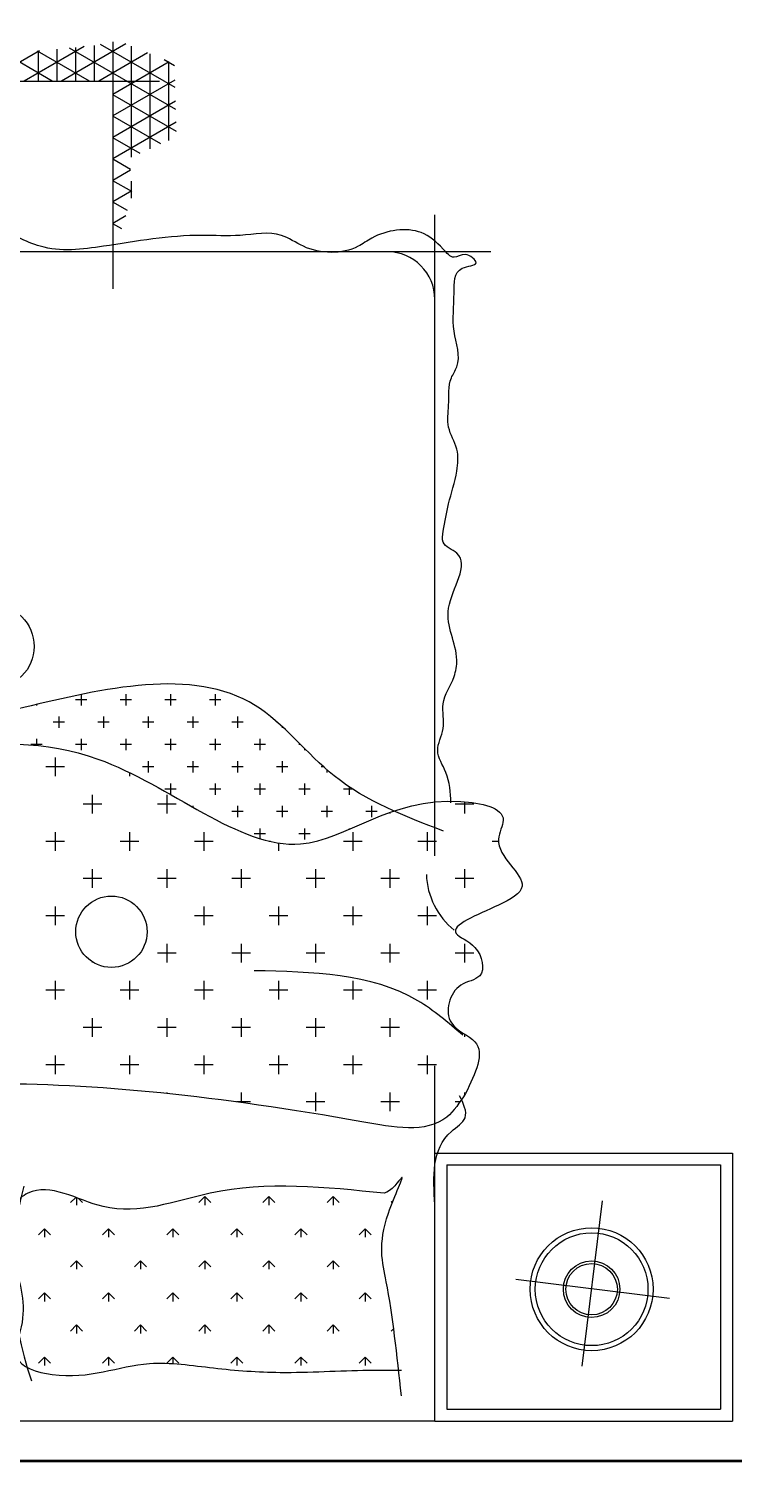
# Model space of a CAD drawing. Units: inches. Extents: x 3731 to 4318, y 1310 to 2388.
# Tile 13 of 57: x 4038 to 4086, y 1363 to 1463. Entities that reach past the tile are written whole.
import ezdxf

# ---------------------------------------------------------------- set-up
doc = ezdxf.new("R2010")
doc.units = ezdxf.units.IN
for name, color, linetype, lineweight in [('A-ANNO-DIMS', 2, 'Continuous', 18), ('A-FURN', 8, 'Continuous', 13), ('A-WALL', 7, 'Continuous', 35)]:
    doc.layers.add(name, color=color, linetype=linetype, lineweight=lineweight)
doc.styles.get("Standard").update_dxf_attribs({"font": 'arial.ttf'})
doc.dimstyles.get("Standard").update_dxf_attribs({"dimtxt": 0.18, "dimasz": 0.18, "dimexe": 0.18, "dimexo": 0.0625, "dimgap": 0.09, "dimtad": 0, "dimtih": 1, "dimtoh": 1, "dimdec": 4, "dimzin": 0, "dimdsep": 46, "dimtxsty": 'Standard', "dimcen": 0.09, "dimadec": 0, "dimazin": 0, "dimtfac": 1, "dimtdec": 4, "dimtofl": 0, "dimtmove": 0, "dimatfit": 3, "dimfxl": 1, "dimtolj": 1, "dimtzin": 0, "dimarcsym": 0})

# ---------------------------------------------------------------- blocks, each defined once
blk = doc.blocks.new('A$C200C7901')
for p, q in [((0, 1.8834), (0, 2.3334)), ((0.5, 2.3334), (0, 2.3334)), ((0.5, 2.3334), (0.5, 1.7369)), ((0.5, 2.3334), (0.5, 1.7369)), ((0.5, 2.3334), (2, 2.3334)), ((0.9943, 2.1721), (0.9842, 2.1822)), ((0.9943, 2.1721), (0.9842, 2.1822)), ((0.9943, 2.0643), (0.9842, 2.0744)), ((0.9943, 2.0643), (0.9842, 2.0744)), ((0.5701, 1.9635), (0.5733, 1.9666)), ((0.5701, 1.9635), (0.5733, 1.9666)), ((0.5, 1.8834), (0, 1.8834)), ((0.4504, 1.782), (0.4504, 1.7863)), ((0.4504, 1.782), (0.4504, 1.7863)), ((0.458, 1.7977), (0.466, 1.7977)), ((0.458, 1.7977), (0.466, 1.7977)), ((1.1222, 1.7352), (1.1535, 1.7352)), ((1.1379, 1.7195), (1.1379, 1.7508)), ((0.4504, 1.6834), (0.4504, 1.6883)), ((0.4504, 1.6834), (0.4504, 1.6883)), ((0.4656, 1.6727), (0.466, 1.6727)), ((0.4656, 1.6727), (0.466, 1.6727)), ((0.5597, 1.6727), (0.591, 1.6727)), ((0.5597, 1.6727), (0.591, 1.6727)), ((1.0129, 1.5945), (1.0129, 1.6258)), ((1.0129, 1.5945), (1.0129, 1.6258)), ((0.4504, 1.532), (0.4504, 1.5633)), ((1.0754, 1.5625), (1.0754, 1.5633)), ((1.0754, 1.5625), (1.0754, 1.5633)), ((0.4347, 1.5477), (0.466, 1.5477)), ((0.6847, 1.5477), (0.716, 1.5477)), ((0.4347, 1.4227), (0.466, 1.4227)), ((0.5, 1.3845), (0.5, 0.3086)), ((0.3931, 1.3602), (0.4035, 1.3602)), ((0.3931, 1.3602), (0.4035, 1.3602)), ((0.4972, 1.3602), (0.5285, 1.3602)), ((0.4972, 1.3602), (0.5285, 1.3602)), ((0.4347, 1.2977), (0.466, 1.2977)), ((0.4347, 1.2977), (0.466, 1.2977)), ((0.4504, 1.2936), (0.4504, 1.3133)), ((0.4504, 1.2936), (0.4504, 1.3133)), ((1.0407, 0.0275), (1.0407, 0.4323)), ((0.4061, 0.3703), (2.0386, 0.3703)), ((2.4073, 0.0839), (0.9625, 0.0839))]:
    blk.add_line(p, q)
at = {"linetype": 'ByBlock'}
for p, q in [((0.02, 1.9034), (0.02, 2.3134)), ((0.48, 2.3134), (0.02, 2.3134)), ((0.48, 1.9034), (0.48, 2.3134)), ((0.2524, 2.2412), (0.2186, 1.9635)), ((0.6171, 2.2259), (0.607, 2.236)), ((0.6171, 2.2259), (0.607, 2.236)), ((0.6171, 2.2259), (0.6171, 2.2402)), ((0.6171, 2.2259), (0.6171, 2.2402)), ((0.6171, 2.2259), (0.6272, 2.236)), ((0.6171, 2.2259), (0.6272, 2.236)), ((0.7249, 2.2259), (0.7148, 2.236)), ((0.7249, 2.2259), (0.7148, 2.236)), ((0.7249, 2.2259), (0.7249, 2.2402)), ((0.7249, 2.2259), (0.7249, 2.2402)), ((0.7249, 2.2259), (0.735, 2.236)), ((0.7249, 2.2259), (0.735, 2.236)), ((0.8326, 2.2259), (0.8225, 2.236)), ((0.8326, 2.2259), (0.8225, 2.236)), ((0.8326, 2.2259), (0.8326, 2.2402)), ((0.8326, 2.2259), (0.8326, 2.2402)), ((0.8326, 2.2259), (0.8427, 2.236)), ((0.8326, 2.2259), (0.8427, 2.236)), ((0.9404, 2.2259), (0.9303, 2.236)), ((0.9404, 2.2259), (0.9303, 2.236)), ((0.9404, 2.2259), (0.9404, 2.2369)), ((0.9404, 2.2259), (0.9404, 2.2369)), ((0.9404, 2.2259), (0.9505, 2.236)), ((0.9404, 2.2259), (0.9505, 2.236)), ((1.0482, 2.2259), (1.0381, 2.236)), ((1.0482, 2.2259), (1.0381, 2.236)), ((1.0482, 2.2259), (1.0482, 2.2402)), ((1.0482, 2.2259), (1.0482, 2.2402)), ((1.0482, 2.2259), (1.0583, 2.236)), ((1.0482, 2.2259), (1.0583, 2.236)), ((1.1559, 2.2259), (1.1458, 2.236)), ((1.1559, 2.2259), (1.1458, 2.236)), ((1.1559, 2.2259), (1.1559, 2.2402)), ((1.1559, 2.2259), (1.1559, 2.2402)), ((1.1559, 2.2259), (1.166, 2.236)), ((1.1559, 2.2259), (1.166, 2.236)), ((0.5692, 2.178), (0.5733, 2.1822)), ((0.5692, 2.178), (0.5733, 2.1822)), ((0.671, 2.1721), (0.6609, 2.1822)), ((0.671, 2.1721), (0.6609, 2.1822)), ((0.671, 2.172), (0.671, 2.1863)), ((0.671, 2.172), (0.671, 2.1863)), ((0.671, 2.1721), (0.6811, 2.1822)), ((0.671, 2.1721), (0.6811, 2.1822)), ((0.7787, 2.1721), (0.7686, 2.1822)), ((0.7787, 2.1721), (0.7686, 2.1822)), ((0.7787, 2.172), (0.7787, 2.1863)), ((0.7787, 2.172), (0.7787, 2.1863)), ((0.7787, 2.1721), (0.7889, 2.1822)), ((0.7787, 2.1721), (0.7889, 2.1822)), ((0.8865, 2.1721), (0.8764, 2.1822)), ((0.8865, 2.1721), (0.8764, 2.1822)), ((0.8865, 2.172), (0.8865, 2.1863)), ((0.8865, 2.172), (0.8865, 2.1863)), ((0.8865, 2.1721), (0.8966, 2.1822)), ((0.8865, 2.1721), (0.8966, 2.1822)), ((0.9943, 2.172), (0.9943, 2.1863)), ((0.9943, 2.172), (0.9943, 2.1863)), ((0.9943, 2.1721), (1.0044, 2.1822)), ((0.9943, 2.1721), (1.0044, 2.1822)), ((1.102, 2.1721), (1.0919, 2.1822)), ((1.102, 2.1721), (1.0919, 2.1822)), ((1.102, 2.172), (1.102, 2.1863)), ((1.102, 2.172), (1.102, 2.1863)), ((1.102, 2.1721), (1.1121, 2.1822)), ((1.102, 2.1721), (1.1121, 2.1822)), ((0.3641, 2.0951), (0.1061, 2.1268)), ((0.6171, 2.1182), (0.607, 2.1283)), ((0.6171, 2.1182), (0.607, 2.1283)), ((0.6171, 2.1182), (0.6171, 2.1325)), ((0.6171, 2.1182), (0.6171, 2.1325)), ((0.6171, 2.1182), (0.6272, 2.1283)), ((0.6171, 2.1182), (0.6272, 2.1283)), ((0.7249, 2.1182), (0.7148, 2.1283)), ((0.7249, 2.1182), (0.7148, 2.1283)), ((0.7249, 2.1182), (0.7249, 2.1325)), ((0.7249, 2.1182), (0.7249, 2.1325)), ((0.7249, 2.1182), (0.735, 2.1283)), ((0.7249, 2.1182), (0.735, 2.1283)), ((0.8326, 2.1182), (0.8225, 2.1283)), ((0.8326, 2.1182), (0.8225, 2.1283)), ((0.8326, 2.1182), (0.8326, 2.1325)), ((0.8326, 2.1182), (0.8326, 2.1325)), ((0.8326, 2.1182), (0.8427, 2.1283)), ((0.8326, 2.1182), (0.8427, 2.1283)), ((0.9404, 2.1182), (0.9303, 2.1283)), ((0.9404, 2.1182), (0.9303, 2.1283)), ((0.9404, 2.1182), (0.9404, 2.1325)), ((0.9404, 2.1182), (0.9404, 2.1325)), ((0.9404, 2.1182), (0.9505, 2.1283)), ((0.9404, 2.1182), (0.9505, 2.1283)), ((1.0482, 2.1182), (1.0381, 2.1283)), ((1.0482, 2.1182), (1.0381, 2.1283)), ((1.0482, 2.1182), (1.0482, 2.1325)), ((1.0482, 2.1182), (1.0482, 2.1325)), ((1.0482, 2.1182), (1.0583, 2.1283)), ((1.0482, 2.1182), (1.0583, 2.1283)), ((1.1559, 2.1182), (1.1458, 2.1283)), ((1.1559, 2.1182), (1.1458, 2.1283)), ((1.1559, 2.1182), (1.1559, 2.1325)), ((1.1559, 2.1182), (1.1559, 2.1325)), ((1.1559, 2.1182), (1.166, 2.1283)), ((1.1559, 2.1182), (1.166, 2.1283)), ((0.671, 2.0643), (0.671, 2.0786)), ((0.671, 2.0643), (0.671, 2.0786)), ((0.7787, 2.0643), (0.7787, 2.0786)), ((0.7787, 2.0643), (0.7787, 2.0786)), ((0.8865, 2.0643), (0.8865, 2.0786)), ((0.8865, 2.0643), (0.8865, 2.0786)), ((0.9943, 2.0643), (0.9943, 2.0786)), ((0.9943, 2.0643), (0.9943, 2.0786)), ((1.102, 2.0643), (1.102, 2.0786)), ((1.102, 2.0643), (1.102, 2.0786)), ((0.671, 2.0643), (0.6609, 2.0744)), ((0.671, 2.0643), (0.6609, 2.0744)), ((0.671, 2.0643), (0.6811, 2.0744)), ((0.671, 2.0643), (0.6811, 2.0744)), ((0.7787, 2.0643), (0.7686, 2.0744)), ((0.7787, 2.0643), (0.7686, 2.0744)), ((0.7787, 2.0643), (0.7889, 2.0744)), ((0.7787, 2.0643), (0.7889, 2.0744)), ((0.8865, 2.0643), (0.8764, 2.0744)), ((0.8865, 2.0643), (0.8764, 2.0744)), ((0.8865, 2.0643), (0.8966, 2.0744)), ((0.8865, 2.0643), (0.8966, 2.0744)), ((0.9943, 2.0643), (1.0044, 2.0744)), ((0.9943, 2.0643), (1.0044, 2.0744)), ((1.102, 2.0643), (1.0919, 2.0744)), ((1.102, 2.0643), (1.0919, 2.0744)), ((1.102, 2.0643), (1.1121, 2.0744)), ((1.102, 2.0643), (1.1121, 2.0744)), ((0.6171, 2.0104), (0.607, 2.0205)), ((0.6171, 2.0104), (0.607, 2.0205)), ((0.6171, 2.0104), (0.6171, 2.0247)), ((0.6171, 2.0104), (0.6171, 2.0247)), ((0.6171, 2.0104), (0.6272, 2.0205)), ((0.6171, 2.0104), (0.6272, 2.0205)), ((0.7249, 2.0104), (0.7148, 2.0205)), ((0.7249, 2.0104), (0.7148, 2.0205)), ((0.7249, 2.0104), (0.7249, 2.0247)), ((0.7249, 2.0104), (0.7249, 2.0247)), ((0.7249, 2.0104), (0.735, 2.0205)), ((0.7249, 2.0104), (0.735, 2.0205)), ((0.8326, 2.0104), (0.8225, 2.0205)), ((0.8326, 2.0104), (0.8225, 2.0205)), ((0.8326, 2.0104), (0.8326, 2.0247)), ((0.8326, 2.0104), (0.8326, 2.0247)), ((0.8326, 2.0104), (0.8427, 2.0205)), ((0.8326, 2.0104), (0.8427, 2.0205)), ((0.9404, 2.0104), (0.9303, 2.0205)), ((0.9404, 2.0104), (0.9303, 2.0205)), ((0.9404, 2.0104), (0.9404, 2.0247)), ((0.9404, 2.0104), (0.9404, 2.0247)), ((0.9404, 2.0104), (0.9505, 2.0205)), ((0.9404, 2.0104), (0.9505, 2.0205)), ((1.0482, 2.0104), (1.0381, 2.0205)), ((1.0482, 2.0104), (1.0381, 2.0205)), ((1.0482, 2.0104), (1.0482, 2.0247)), ((1.0482, 2.0104), (1.0482, 2.0247)), ((1.0482, 2.0104), (1.0583, 2.0205)), ((1.0482, 2.0104), (1.0583, 2.0205)), ((1.1559, 2.0104), (1.1458, 2.0205)), ((1.1559, 2.0104), (1.1458, 2.0205)), ((1.1559, 2.0104), (1.1559, 2.0247)), ((1.1559, 2.0104), (1.1559, 2.0247)), ((1.1559, 2.0104), (1.166, 2.0205)), ((1.1559, 2.0104), (1.166, 2.0205)), ((0.671, 1.9565), (0.6609, 1.9666)), ((0.671, 1.9565), (0.6609, 1.9666)), ((0.671, 1.9565), (0.671, 1.9708)), ((0.671, 1.9565), (0.671, 1.9708)), ((0.671, 1.9565), (0.6811, 1.9666)), ((0.671, 1.9565), (0.6811, 1.9666)), ((0.7787, 1.9565), (0.7686, 1.9666)), ((0.7787, 1.9565), (0.7686, 1.9666)), ((0.7787, 1.9565), (0.7787, 1.9708)), ((0.7787, 1.9565), (0.7787, 1.9708)), ((0.7787, 1.9565), (0.7889, 1.9666)), ((0.7787, 1.9565), (0.7889, 1.9666)), ((0.8865, 1.9565), (0.8764, 1.9666)), ((0.8865, 1.9565), (0.8764, 1.9666)), ((0.8865, 1.9565), (0.8865, 1.9708)), ((0.8865, 1.9565), (0.8865, 1.9708)), ((0.8865, 1.9565), (0.8966, 1.9666)), ((0.8865, 1.9565), (0.8966, 1.9666)), ((1.0993, 1.9593), (1.0919, 1.9666)), ((1.0993, 1.9593), (1.0919, 1.9666)), ((1.102, 1.9583), (1.102, 1.9708)), ((1.102, 1.9583), (1.102, 1.9708)), ((1.1033, 1.9578), (1.1121, 1.9666)), ((1.1033, 1.9578), (1.1121, 1.9666)), ((0.48, 1.9034), (0.02, 1.9034)), ((0.5754, 1.782), (0.5754, 1.8133)), ((0.5754, 1.782), (0.5754, 1.8133)), ((0.7004, 1.782), (0.7004, 1.8133)), ((0.7004, 1.782), (0.7004, 1.8133)), ((0.5597, 1.7977), (0.591, 1.7977)), ((0.5597, 1.7977), (0.591, 1.7977)), ((0.6847, 1.7977), (0.716, 1.7977)), ((0.6847, 1.7977), (0.716, 1.7977)), ((0.8097, 1.7977), (0.8331, 1.7977)), ((0.8097, 1.7977), (0.8331, 1.7977)), ((0.8254, 1.782), (0.8254, 1.7987)), ((0.8254, 1.782), (0.8254, 1.7987)), ((0.9504, 1.782), (0.9504, 1.7836)), ((0.9504, 1.782), (0.9504, 1.7836)), ((0.4972, 1.7352), (0.5285, 1.7352)), ((0.4972, 1.7352), (0.5285, 1.7352)), ((0.5129, 1.7195), (0.5129, 1.7508)), ((0.5129, 1.7195), (0.5129, 1.7508)), ((0.6222, 1.7352), (0.6535, 1.7352)), ((0.6222, 1.7352), (0.6535, 1.7352)), ((0.6379, 1.7195), (0.6379, 1.7508)), ((0.6379, 1.7195), (0.6379, 1.7508)), ((0.7472, 1.7352), (0.7785, 1.7352)), ((0.7472, 1.7352), (0.7785, 1.7352)), ((0.7629, 1.7195), (0.7629, 1.7508)), ((0.7629, 1.7195), (0.7629, 1.7508)), ((0.8722, 1.7352), (0.9035, 1.7352)), ((0.8722, 1.7352), (0.9035, 1.7352)), ((0.8879, 1.7195), (0.8879, 1.7508)), ((0.8879, 1.7195), (0.8879, 1.7508)), ((0.9972, 1.7352), (1.0285, 1.7352)), ((0.9972, 1.7352), (1.0285, 1.7352)), ((1.0129, 1.7195), (1.0129, 1.7508)), ((1.0129, 1.7195), (1.0129, 1.7508)), ((1.1222, 1.7352), (1.1535, 1.7352)), ((1.1379, 1.7195), (1.1379, 1.7508)), ((0.5754, 1.657), (0.5754, 1.6883)), ((0.5754, 1.657), (0.5754, 1.6883)), ((0.7004, 1.657), (0.7004, 1.6883)), ((0.7004, 1.657), (0.7004, 1.6883)), ((0.8254, 1.657), (0.8254, 1.6883)), ((0.8254, 1.657), (0.8254, 1.6883)), ((0.9504, 1.657), (0.9504, 1.6883)), ((0.9504, 1.657), (0.9504, 1.6883)), ((1.0754, 1.657), (1.0754, 1.6883)), ((1.0754, 1.657), (1.0754, 1.6883)), ((0.6847, 1.6727), (0.716, 1.6727)), ((0.6847, 1.6727), (0.716, 1.6727)), ((0.8097, 1.6727), (0.841, 1.6727)), ((0.8097, 1.6727), (0.841, 1.6727)), ((0.9347, 1.6727), (0.966, 1.6727)), ((0.9347, 1.6727), (0.966, 1.6727)), ((1.0597, 1.6727), (1.091, 1.6727)), ((1.0597, 1.6727), (1.091, 1.6727)), ((0.5129, 1.5945), (0.5129, 1.6258)), ((0.5129, 1.5945), (0.5129, 1.6258)), ((0.6379, 1.5945), (0.6379, 1.6258)), ((0.6379, 1.5945), (0.6379, 1.6258)), ((0.7629, 1.5945), (0.7629, 1.6258)), ((0.7629, 1.5945), (0.7629, 1.6258)), ((0.8879, 1.5945), (0.8879, 1.6258)), ((0.8879, 1.5945), (0.8879, 1.6258)), ((1.1379, 1.5945), (1.1379, 1.6258)), ((1.1379, 1.5945), (1.1379, 1.6258)), ((0.4972, 1.6102), (0.5285, 1.6102)), ((0.4972, 1.6102), (0.5285, 1.6102)), ((0.6222, 1.6102), (0.6535, 1.6102)), ((0.6222, 1.6102), (0.6535, 1.6102)), ((0.7472, 1.6102), (0.7785, 1.6102)), ((0.7472, 1.6102), (0.7785, 1.6102)), ((0.8722, 1.6102), (0.9035, 1.6102)), ((0.8722, 1.6102), (0.9035, 1.6102)), ((0.9972, 1.6102), (1.0285, 1.6102)), ((0.9972, 1.6102), (1.0285, 1.6102)), ((1.1222, 1.6102), (1.1535, 1.6102)), ((1.1222, 1.6102), (1.1535, 1.6102)), ((0.4504, 1.532), (0.4504, 1.5633)), ((0.5754, 1.532), (0.5754, 1.5633)), ((0.5754, 1.532), (0.5754, 1.5633)), ((0.7004, 1.532), (0.7004, 1.5633)), ((0.7004, 1.532), (0.7004, 1.5633)), ((0.8254, 1.532), (0.8254, 1.5633)), ((0.8254, 1.532), (0.8254, 1.5633)), ((0.9504, 1.532), (0.9504, 1.5633)), ((0.9504, 1.532), (0.9504, 1.5633)), ((0.4347, 1.5477), (0.466, 1.5477)), ((0.5597, 1.5477), (0.591, 1.5477)), ((0.5597, 1.5477), (0.591, 1.5477)), ((0.6847, 1.5477), (0.716, 1.5477)), ((0.8097, 1.5477), (0.841, 1.5477)), ((0.8097, 1.5477), (0.841, 1.5477)), ((0.9347, 1.5477), (0.966, 1.5477)), ((0.9347, 1.5477), (0.966, 1.5477)), ((0.5129, 1.4695), (0.5129, 1.5008)), ((0.5129, 1.4695), (0.5129, 1.5008)), ((0.6379, 1.4695), (0.6379, 1.5008)), ((0.6379, 1.4695), (0.6379, 1.5008)), ((0.7629, 1.4695), (0.7629, 1.5008)), ((0.7629, 1.4695), (0.7629, 1.5008)), ((0.8879, 1.4695), (0.8879, 1.5008)), ((0.8879, 1.4695), (0.8879, 1.5008)), ((1.1379, 1.4695), (1.1379, 1.5008)), ((1.1379, 1.4695), (1.1379, 1.5008)), ((0.4972, 1.4852), (0.5285, 1.4852)), ((0.4972, 1.4852), (0.5285, 1.4852)), ((0.6222, 1.4852), (0.6535, 1.4852)), ((0.6222, 1.4852), (0.6535, 1.4852)), ((0.7472, 1.4852), (0.7785, 1.4852)), ((0.7472, 1.4852), (0.7785, 1.4852)), ((0.8722, 1.4852), (0.9035, 1.4852)), ((0.8722, 1.4852), (0.9035, 1.4852)), ((1.1222, 1.4852), (1.1535, 1.4852)), ((1.1222, 1.4852), (1.1535, 1.4852)), ((0.4347, 1.4227), (0.466, 1.4227)), ((0.4504, 1.407), (0.4504, 1.4383)), ((0.4504, 1.407), (0.4504, 1.4383)), ((0.5597, 1.4227), (0.591, 1.4227)), ((0.5597, 1.4227), (0.591, 1.4227)), ((0.5754, 1.407), (0.5754, 1.4383)), ((0.5754, 1.407), (0.5754, 1.4383)), ((0.6847, 1.4227), (0.716, 1.4227)), ((0.6847, 1.4227), (0.716, 1.4227)), ((0.7004, 1.407), (0.7004, 1.4383)), ((0.7004, 1.407), (0.7004, 1.4383)), ((0.8097, 1.4227), (0.841, 1.4227)), ((0.8097, 1.4227), (0.841, 1.4227)), ((0.8254, 1.407), (0.8254, 1.4383)), ((0.8254, 1.407), (0.8254, 1.4383)), ((0.9347, 1.4227), (0.966, 1.4227)), ((0.9347, 1.4227), (0.966, 1.4227)), ((0.9504, 1.407), (0.9504, 1.4383)), ((0.9504, 1.407), (0.9504, 1.4383)), ((1.0597, 1.4227), (1.091, 1.4227)), ((1.0597, 1.4227), (1.091, 1.4227)), ((1.0754, 1.407), (1.0754, 1.4383)), ((1.0754, 1.407), (1.0754, 1.4383)), ((0.5129, 1.3445), (0.5129, 1.3758)), ((0.5129, 1.3445), (0.5129, 1.3758)), ((0.6379, 1.3445), (0.6379, 1.3758)), ((0.6379, 1.3445), (0.6379, 1.3758)), ((0.7629, 1.3627), (0.7629, 1.3758)), ((0.7629, 1.3627), (0.7629, 1.3758)), ((0.8879, 1.3445), (0.8879, 1.3758)), ((0.8879, 1.3445), (0.8879, 1.3758)), ((1.0129, 1.3445), (1.0129, 1.3758)), ((1.0129, 1.3445), (1.0129, 1.3758)), ((1.1379, 1.3445), (1.1379, 1.3758)), ((1.1379, 1.3445), (1.1379, 1.3758)), ((0.6222, 1.3602), (0.6535, 1.3602)), ((0.6222, 1.3602), (0.6535, 1.3602)), ((0.7097, 1.3477), (0.7285, 1.3477)), ((0.7097, 1.3477), (0.7285, 1.3477)), ((0.7191, 1.3383), (0.7191, 1.357)), ((0.7191, 1.3383), (0.7191, 1.357)), ((0.7762, 1.3602), (0.7785, 1.3602)), ((0.7762, 1.3602), (0.7785, 1.3602)), ((0.7847, 1.3477), (0.8035, 1.3477)), ((0.7847, 1.3477), (0.8035, 1.3477)), ((0.7941, 1.3383), (0.7941, 1.3554)), ((0.7941, 1.3383), (0.7941, 1.3554)), ((0.8722, 1.3602), (0.9035, 1.3602)), ((0.8722, 1.3602), (0.9035, 1.3602)), ((0.9972, 1.3602), (1.0285, 1.3602)), ((0.9972, 1.3602), (1.0285, 1.3602)), ((1.1222, 1.3602), (1.1535, 1.3602)), ((1.1222, 1.3602), (1.1535, 1.3602)), ((0.6066, 1.3008), (0.6066, 1.3195)), ((0.6066, 1.3008), (0.6066, 1.3195)), ((0.6441, 1.3383), (0.6441, 1.3399)), ((0.6441, 1.3383), (0.6441, 1.3399)), ((0.6816, 1.3008), (0.6816, 1.3195)), ((0.6816, 1.3008), (0.6816, 1.3195)), ((0.7566, 1.3008), (0.7566, 1.3195)), ((0.7566, 1.3008), (0.7566, 1.3195)), ((0.8316, 1.3008), (0.8316, 1.3195)), ((0.8316, 1.3008), (0.8316, 1.3195)), ((0.5754, 1.3115), (0.5754, 1.3133)), ((0.5754, 1.3115), (0.5754, 1.3133)), ((0.5972, 1.3102), (0.616, 1.3102)), ((0.5972, 1.3102), (0.616, 1.3102)), ((0.6722, 1.3102), (0.691, 1.3102)), ((0.6722, 1.3102), (0.691, 1.3102)), ((0.7472, 1.3102), (0.766, 1.3102)), ((0.7472, 1.3102), (0.766, 1.3102)), ((0.8222, 1.3102), (0.841, 1.3102)), ((0.8222, 1.3102), (0.841, 1.3102)), ((0.9066, 1.3008), (0.9066, 1.3028)), ((0.9066, 1.3008), (0.9066, 1.3028)), ((0.9347, 1.2977), (0.966, 1.2977)), ((0.9347, 1.2977), (0.966, 1.2977)), ((0.9504, 1.282), (0.9504, 1.3133)), ((0.9504, 1.282), (0.9504, 1.3133)), ((1.0597, 1.2977), (1.091, 1.2977)), ((1.0597, 1.2977), (1.091, 1.2977)), ((1.0754, 1.282), (1.0754, 1.3133)), ((1.0754, 1.282), (1.0754, 1.3133)), ((0.6379, 1.2727), (0.6535, 1.2727)), ((0.6379, 1.2727), (0.6535, 1.2727)), ((0.6441, 1.2686), (0.6441, 1.282)), ((0.6441, 1.2686), (0.6441, 1.282)), ((0.7097, 1.2727), (0.7285, 1.2727)), ((0.7097, 1.2727), (0.7285, 1.2727)), ((0.7191, 1.2633), (0.7191, 1.282)), ((0.7191, 1.2633), (0.7191, 1.282)), ((0.7847, 1.2727), (0.8035, 1.2727)), ((0.7847, 1.2727), (0.8035, 1.2727)), ((0.7941, 1.2633), (0.7941, 1.282)), ((0.7941, 1.2633), (0.7941, 1.282)), ((0.8597, 1.2727), (0.8785, 1.2727)), ((0.8597, 1.2727), (0.8785, 1.2727)), ((0.8691, 1.2633), (0.8691, 1.282)), ((0.8691, 1.2633), (0.8691, 1.282)), ((0.9347, 1.2727), (0.9535, 1.2727)), ((0.9347, 1.2727), (0.9535, 1.2727)), ((0.9441, 1.2633), (0.9441, 1.2816)), ((0.9441, 1.2633), (0.9441, 1.2816)), ((1.0129, 1.2448), (1.0129, 1.2508)), ((1.0129, 1.2448), (1.0129, 1.2508)), ((1.1379, 1.2195), (1.1379, 1.2508)), ((1.1379, 1.2195), (1.1379, 1.2508)), ((0.6816, 1.2398), (0.6816, 1.2445)), ((0.6816, 1.2398), (0.6816, 1.2445)), ((0.6868, 1.2352), (0.691, 1.2352)), ((0.6868, 1.2352), (0.691, 1.2352)), ((0.7472, 1.2352), (0.766, 1.2352)), ((0.7472, 1.2352), (0.766, 1.2352)), ((0.7566, 1.2258), (0.7566, 1.2445)), ((0.7566, 1.2258), (0.7566, 1.2445)), ((0.8222, 1.2352), (0.841, 1.2352)), ((0.8222, 1.2352), (0.841, 1.2352)), ((0.8316, 1.2258), (0.8316, 1.2445)), ((0.8316, 1.2258), (0.8316, 1.2445)), ((0.8972, 1.2352), (0.916, 1.2352)), ((0.8972, 1.2352), (0.916, 1.2352)), ((0.9066, 1.2258), (0.9066, 1.2445)), ((0.9066, 1.2258), (0.9066, 1.2445)), ((0.9722, 1.2352), (0.991, 1.2352)), ((0.9722, 1.2352), (0.991, 1.2352)), ((0.9816, 1.2258), (0.9816, 1.2445)), ((0.9816, 1.2258), (0.9816, 1.2445)), ((1.1222, 1.2352), (1.1535, 1.2352)), ((1.1222, 1.2352), (1.1535, 1.2352)), ((0.7191, 1.2041), (0.7191, 1.207)), ((0.7191, 1.2041), (0.7191, 1.207)), ((0.7255, 1.1977), (0.7285, 1.1977)), ((0.7255, 1.1977), (0.7285, 1.1977)), ((0.7847, 1.1977), (0.8035, 1.1977)), ((0.7847, 1.1977), (0.8035, 1.1977)), ((0.7941, 1.1883), (0.7941, 1.207)), ((0.7941, 1.1883), (0.7941, 1.207)), ((0.8597, 1.1977), (0.8785, 1.1977)), ((0.8597, 1.1977), (0.8785, 1.1977)), ((0.8691, 1.1883), (0.8691, 1.207)), ((0.8691, 1.1883), (0.8691, 1.207)), ((0.9347, 1.1977), (0.9535, 1.1977)), ((0.9347, 1.1977), (0.9535, 1.1977)), ((0.9441, 1.1883), (0.9441, 1.207)), ((0.9441, 1.1883), (0.9441, 1.207)), ((1.0097, 1.1977), (1.0285, 1.1977)), ((1.0097, 1.1977), (1.0285, 1.1977)), ((1.0191, 1.1883), (1.0191, 1.207)), ((1.0191, 1.1883), (1.0191, 1.207)), ((1.0847, 1.1977), (1.1035, 1.1977)), ((1.0847, 1.1977), (1.1035, 1.1977)), ((1.0941, 1.1883), (1.0941, 1.207)), ((1.0941, 1.1883), (1.0941, 1.207)), ((1.1597, 1.1977), (1.1785, 1.1977)), ((1.1597, 1.1977), (1.1785, 1.1977)), ((1.1691, 1.1883), (1.1691, 1.1991)), ((1.1691, 1.1883), (1.1691, 1.1991)), ((0.7566, 1.1674), (0.7566, 1.1695)), ((0.7566, 1.1674), (0.7566, 1.1695)), ((0.7646, 1.1602), (0.766, 1.1602)), ((0.7646, 1.1602), (0.766, 1.1602)), ((0.8222, 1.1602), (0.841, 1.1602)), ((0.8222, 1.1602), (0.841, 1.1602)), ((0.8316, 1.1508), (0.8316, 1.1695)), ((0.8316, 1.1508), (0.8316, 1.1695)), ((0.8972, 1.1602), (0.916, 1.1602)), ((0.8972, 1.1602), (0.916, 1.1602)), ((0.9066, 1.1508), (0.9066, 1.1695)), ((0.9066, 1.1508), (0.9066, 1.1695)), ((0.9722, 1.1602), (0.991, 1.1602)), ((0.9722, 1.1602), (0.991, 1.1602)), ((0.9816, 1.1508), (0.9816, 1.1695)), ((0.9816, 1.1508), (0.9816, 1.1695)), ((1.0472, 1.1602), (1.066, 1.1602)), ((1.0472, 1.1602), (1.066, 1.1602)), ((1.0566, 1.1508), (1.0566, 1.1695)), ((1.0566, 1.1508), (1.0566, 1.1695)), ((1.1222, 1.1602), (1.141, 1.1602)), ((1.1222, 1.1602), (1.141, 1.1602)), ((1.1316, 1.1508), (1.1316, 1.1695)), ((1.1316, 1.1508), (1.1316, 1.1695)), ((0.8691, 1.1133), (0.8691, 1.132)), ((0.8691, 1.1133), (0.8691, 1.132)), ((0.9441, 1.1133), (0.9441, 1.132)), ((0.9441, 1.1133), (0.9441, 1.132)), ((1.0191, 1.1133), (1.0191, 1.132)), ((1.0191, 1.1133), (1.0191, 1.132)), ((1.0941, 1.1136), (1.0941, 1.132)), ((1.0941, 1.1136), (1.0941, 1.132)), ((1.1691, 1.1303), (1.1691, 1.132)), ((1.1691, 1.1303), (1.1691, 1.132)), ((0.8597, 1.1227), (0.8785, 1.1227)), ((0.8597, 1.1227), (0.8785, 1.1227)), ((0.9347, 1.1227), (0.9535, 1.1227)), ((0.9347, 1.1227), (0.9535, 1.1227)), ((1.0097, 1.1227), (1.0285, 1.1227)), ((1.0097, 1.1227), (1.0285, 1.1227)), ((1.0847, 1.1227), (1.1035, 1.1227)), ((1.0847, 1.1227), (1.1035, 1.1227)), ((1.0194, 0.3103), (1.0407, 0.3227)), ((1.0194, 0.3103), (1.0407, 0.3227)), ((1.0261, 0.3316), (1.0407, 0.3232)), ((1.0261, 0.3316), (1.0407, 0.3232)), ((1.0164, 0.3011), (1.0407, 0.2871)), ((1.0164, 0.3011), (1.0407, 0.2871)), ((1.0088, 0.2694), (1.0407, 0.251)), ((1.0088, 0.2694), (1.0407, 0.251)), ((1.0089, 0.2682), (1.0407, 0.2866)), ((1.0089, 0.2682), (1.0407, 0.2866)), ((1.0099, 0.2521), (1.0099, 0.2804)), ((1.0099, 0.2521), (1.0099, 0.2804)), ((1.0111, 0.2334), (1.0407, 0.2505)), ((1.0111, 0.2334), (1.0407, 0.2505)), ((1.0112, 0.232), (1.0407, 0.215)), ((1.0112, 0.232), (1.0407, 0.215)), ((0.9344, 0.153), (1.0407, 0.2144)), ((0.9344, 0.153), (1.0407, 0.2144)), ((0.9787, 0.0381), (0.9787, 0.1976)), ((0.9787, 0.0381), (0.9787, 0.1976)), ((0.9953, 0.2051), (1.0407, 0.1789)), ((0.9953, 0.2051), (1.0407, 0.1789)), ((1.0099, 0.0251), (1.0099, 0.2117)), ((1.0099, 0.0251), (1.0099, 0.2117)), ((0.9355, 0.1176), (1.0407, 0.1783)), ((0.9355, 0.1176), (1.0407, 0.1783)), ((0.9474, 0.0512), (0.9474, 0.1835)), ((0.9474, 0.0512), (0.9474, 0.1835)), ((0.9602, 0.1893), (1.0407, 0.1428)), ((0.9602, 0.1893), (1.0407, 0.1428)), ((0.9339, 0.1684), (1.0407, 0.1067)), ((0.9339, 0.1684), (1.0407, 0.1067)), ((0.935, 0.1316), (1.114, 0.0283)), ((0.935, 0.1316), (1.114, 0.0283)), ((0.9366, 0.0822), (1.0407, 0.1422)), ((0.9366, 0.0822), (1.0407, 0.1422)), ((0.9463, 0.0516), (1.0407, 0.1061)), ((0.9463, 0.0516), (1.0407, 0.1061)), ((0.9362, 0.0948), (1.0616, 0.0225)), ((0.9362, 0.0948), (1.0616, 0.0225)), ((0.9826, 0.0365), (1.0647, 0.0839)), ((0.9826, 0.0365), (1.0647, 0.0839)), ((1.0189, 0.0214), (1.1272, 0.0839)), ((1.0189, 0.0214), (1.1272, 0.0839)), ((1.0412, 0.0179), (1.0412, 0.0839)), ((1.0412, 0.0179), (1.0412, 0.0839)), ((1.0724, 0.0243), (1.0724, 0.0839)), ((1.0724, 0.0243), (1.0724, 0.0839)), ((1.0801, 0.0839), (1.1675, 0.0335)), ((1.0801, 0.0839), (1.1675, 0.0335)), ((1.0891, 0.0259), (1.1897, 0.0839)), ((1.0891, 0.0259), (1.1897, 0.0839)), ((1.1037, 0.0273), (1.1037, 0.0839)), ((1.1037, 0.0273), (1.1037, 0.0839)), ((1.1349, 0.0303), (1.1349, 0.0839)), ((1.1349, 0.0303), (1.1349, 0.0839)), ((1.1426, 0.0839), (1.2313, 0.0327)), ((1.1426, 0.0839), (1.2313, 0.0327)), ((1.1642, 0.0331), (1.2522, 0.0839)), ((1.1642, 0.0331), (1.2522, 0.0839)), ((1.1662, 0.0333), (1.1662, 0.0839)), ((1.1662, 0.0333), (1.1662, 0.0839)), ((0.9374, 0.0581), (0.9545, 0.0482)), ((0.9374, 0.0581), (0.9545, 0.0482))]:
    blk.add_line(p, q, dxfattribs=at)
for radius in [0.1032, 0.0947, 0.0475, 0.0432]:
    blk.add_circle((0.2367, 2.1121), radius, dxfattribs=at)
for centre, radius in [((1.0433, 1.5119), 0.0599), ((1.2431, 1.0329), 0.0699)]:
    blk.add_circle(centre, radius)
for centre, radius, start, end in [((0.658, 2.0811), 0.5513, 345.0722, 19.5492), ((0.3888, 1.4113), 0.1256, 1.9962, 51.1646), ((0.58, 0.4503), 0.08, 180, 270)]:
    blk.add_arc(centre, radius, start, end)
blk.add_arc((0.3888, 1.4113), 0.1256, 1.9962, 51.1646, dxfattribs=at)
for points, knots in [([(0.5562, 2.2908), (0.5634, 2.223), (0.5751, 2.1147), (0.6005, 2.0213), (0.5392, 1.8966), (0.5726, 1.9486), (0.5854, 1.951)], [0, 0, 0, 0, 193.119101, 308.278592, 371.468985, 410.593498, 410.593498, 410.593498, 410.593498]), ([(0.5854, 1.951), (0.6835, 1.9407), (0.8425, 1.9242), (1.0374, 2.0054), (1.1564, 1.9255), (1.2274, 1.9841), (1.2052, 2.0751), (1.1815, 2.152), (1.2176, 2.2368), (1.0992, 2.2731), (1.0008, 2.2255), (0.8698, 2.246), (0.7481, 2.2548), (0.6426, 2.2473), (0.5746, 2.2478), (0.5562, 2.2479)], [0, 0, 0, 0, 292.165466, 473.33038, 601.631673, 630.723769, 727.138505, 836.819956, 887.958136, 954.42438, 1118.989809, 1227.016542, 1338.750986, 1487.447361, 1542.751028, 1542.751028, 1542.751028, 1542.751028]), ([(0.4485, 1.7835), (0.4321, 1.7496), (0.4062, 1.6964), (0.49, 1.6713), (0.4719, 1.5969), (0.4123, 1.592), (0.4233, 1.5337), (0.4954, 1.5086), (0.4012, 1.4738), (0.3253, 1.4306), (0.4113, 1.3764), (0.3688, 1.3065), (0.5579, 1.2663), (0.741, 1.4533), (1.1127, 1.1109), (1.4811, 1.2478), (1.7885, 1.3492), (2.0357, 1.1637), (2.0748, 1.2974), (2.0876, 1.349), (2.0192, 1.3805), (2.0564, 1.4298), (2.0588, 1.4846), (1.9759, 1.5349), (2.1004, 1.5845), (2.0397, 1.6519), (1.971, 1.7053), (2.1104, 1.8981), (1.5946, 1.7967), (1.2448, 1.7472), (0.8129, 1.7935), (0.4953, 1.8548), (0.4582, 1.7983), (0.4485, 1.7835)], [0, 0, 0, 0, 88.420092, 139.08588, 204.302936, 239.695496, 287.801042, 327.365471, 412.960499, 463.626286, 552.059846, 584.668336, 662.614915, 940.993281, 1309.926334, 1844.022653, 1996.276242, 2316.43048, 2341.441004, 2404.707416, 2449.463774, 2514.680778, 2538.40571, 2613.031547, 2697.13096, 2760.903931, 2822.692699, 2945.47, 3215.060018, 3725.584917, 4361.974444, 4504.671998, 4555.32777, 4555.32777, 4555.32777, 4555.32777]), ([(0.4856, 1.3429), (0.5504, 1.3182), (0.6715, 1.2721), (0.8374, 1.0498), (1.1164, 1.1183), (1.3878, 1.1816), (1.5888, 1.1102), (1.8403, 1.1127), (1.9415, 1.2178), (2.0032, 1.2819)], [0, 0, 0, 0, 205.411753, 383.654933, 772.067458, 921.644661, 1226.793228, 1388.983508, 1642.292305, 1642.292305, 1642.292305, 1642.292305])]:
    blk.add_open_spline(points, degree=3, knots=knots)
for points, knots in [([(0.5, 1.9703), (0.5029, 1.9235), (0.5066, 1.8648), (0.4398, 1.8252), (0.452, 1.8005), (0.4585, 1.7872)], [0, 0, 0, 0, 126.315232, 158.854004, 196.789047, 196.789047, 196.789047, 196.789047]), ([(0.5, 1.9703), (0.5029, 1.9235), (0.5066, 1.8648), (0.4398, 1.8252), (0.452, 1.8005), (0.4585, 1.7872)], [0, 0, 0, 0, 126.315232, 158.854004, 196.789047, 196.789047, 196.789047, 196.789047]), ([(0.4532, 1.6853), (0.4776, 1.6644), (0.574, 1.582), (0.7055, 1.5794), (0.8037, 1.5774)], [0, 0, 0, 0, 94.920667, 374.457292, 374.457292, 374.457292, 374.457292]), ([(0.4532, 1.6853), (0.4776, 1.6644), (0.574, 1.582), (0.7055, 1.5794), (0.8037, 1.5774)], [0, 0, 0, 0, 94.920667, 374.457292, 374.457292, 374.457292, 374.457292]), ([(0.473, 1.2954), (0.4739, 1.2781), (0.4755, 1.2477), (0.5032, 1.2084), (0.4801, 1.1701), (0.4928, 1.1255), (0.4674, 1.0912), (0.4579, 1.0351), (0.501, 0.9724), (0.4311, 0.8832), (0.4902, 0.8637), (0.4843, 0.8288), (0.4774, 0.7906), (0.4625, 0.7457), (0.459, 0.6999), (0.4816, 0.6664), (0.4748, 0.625), (0.4791, 0.5889), (0.4533, 0.5528), (0.4738, 0.5004), (0.4658, 0.4502), (0.4696, 0.3946), (0.4189, 0.3935), (0.4493, 0.3684), (0.4694, 0.3857), (0.4922, 0.3576), (0.5297, 0.3262), (0.5917, 0.3353), (0.6454, 0.3754), (0.7083, 0.3741), (0.7643, 0.3328), (0.826, 0.346), (0.925, 0.3388), (1.0353, 0.3593), (1.1561, 0.3744), (1.2477, 0.3154), (1.3302, 0.3474), (1.4086, 0.3512), (1.5217, 0.3878), (1.6362, 0.3176), (1.7682, 0.3285), (1.8402, 0.3019), (1.9071, 0.3529), (1.9647, 0.3412), (2.0795, 0.2948), (2.0472, 0.3498), (2.0343, 0.3772), (2.0435, 0.43), (2.0109, 0.5782), (2.0746, 0.4643), (2.0805, 0.584), (2.0084, 0.5979), (2.0343, 0.6846), (2.0344, 0.746), (2.0293, 0.8096), (2.0489, 0.8545), (2.0652, 0.9218), (1.9842, 0.9297), (2.0007, 1.0162), (2.0367, 1.0585), (2.0367, 1.1102), (2.0457, 1.1647), (2.0226, 1.2084), (2.0234, 1.2306), (2.0236, 1.2352)], [0, 0, 0, 0, 51.660678, 90.967412, 128.902454, 170.303599, 219.852997, 247.834962, 336.321557, 429.35469, 458.821847, 477.222321, 524.135809, 581.038434, 617.839381, 657.146115, 693.947125, 740.178081, 760.753248, 820.731705, 885.133458, 928.777044, 953.563729, 976.574207, 995.553042, 1018.563482, 1064.584401, 1147.951297, 1174.787598, 1266.851571, 1308.018447, 1377.066427, 1441.511314, 1608.245014, 1714.11869, 1792.771707, 1913.247991, 1954.931389, 2029.864445, 2259.189419, 2305.221512, 2429.507982, 2456.344283, 2543.92595, 2627.925037, 2662.96218, 2687.736879, 2719.937755, 2839.540991, 2875.47895, 2953.681041, 2993.270313, 3066.872333, 3154.395764, 3200.397042, 3248.426375, 3312.828127, 3347.881398, 3444.484026, 3481.577522, 3518.665244, 3592.267265, 3644.719162, 3658.519501, 3658.519501, 3658.519501, 3658.519501])]:
    blk.add_open_spline(points, degree=3, knots=knots, dxfattribs=at)
blk = doc.blocks.new('*D32')
at = {"layer": 'A-ANNO-DIMS', "color": 0, "lineweight": -2, "transparency": 16777216}
for p, q in [((4269.21, 1592.32), (4269.21, 1310.25)), ((3835.21, 1359.32), (3835.21, 1310.25)), ((3835.39, 1310.43), (4051.92, 1310.43)), ((4269.03, 1310.43), (4052.5, 1310.43))]:
    blk.add_line(p, q, dxfattribs=at)
at = {"layer": 'A-ANNO-DIMS', "color": 0, "transparency": 16777216}
for points in [[(3835.39, 1310.46), (3835.39, 1310.4), (3835.21, 1310.43)], [(4269.03, 1310.46), (4269.03, 1310.4), (4269.21, 1310.43)]]:
    blk.add_solid(points, dxfattribs=at)
at = {"layer": 'Defpoints', "color": 0, "transparency": 16777216}
for p in [(4269.21, 1592.38), (3835.21, 1359.38), (4269.21, 1310.43)]:
    blk.add_point(p, dxfattribs=at)
at = {"layer": 'A-ANNO-DIMS', "color": 0, "transparency": 16777216, "insert": (4052.21, 1310.43), "char_height": 0.18, "attachment_point": 5}
blk.add_mtext('\\A1;434', dxfattribs=at)

msp = doc.modelspace()

# ---------------------------------------------------------------- linework, layer by layer
at = {"layer": 'A-WALL'}
msp.add_line((3947.21, 1364.38), (4109.21, 1364.38), dxfattribs=at)

# ---------------------------------------------------------------- block references
at = {"layer": 'A-FURN', "xscale": 41.1071563136412, "yscale": 41.1071563136412, "zscale": 41.1071563136412, "rotation": 180}
msp.add_blockref('A$C200C7901', (4086.15, 1463.04), dxfattribs=at)

# ---------------------------------------------------------------- dimensions: what is measured, and where the dimension line sits
at = {"layer": 'A-ANNO-DIMS'}
dim = msp.add_linear_dim(base=(4269.21, 1310.43), p1=(3835.21, 1359.38), p2=(4269.21, 1592.38), dimstyle='Standard', override={"dimdec": 0, "dimlfac": 1, "dimrnd": 0, "dimzin": 0, "dimdsep": 46, "dimlunit": 2}, dxfattribs=at)
dim.commit()
dim.dimension.update_dxf_attribs({"geometry": '*D32', "text_midpoint": (4052.21, 1310.43)})

doc.saveas('drawing.dxf')
